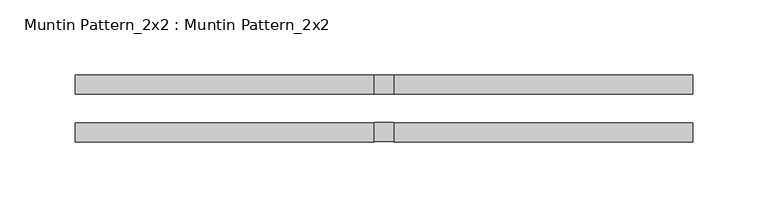
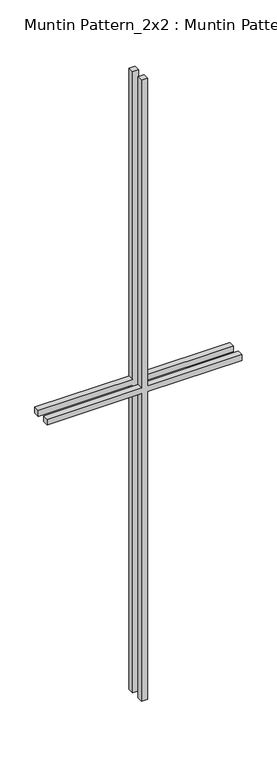
"""IFC4 building model written with IfcOpenShell, lengths in millimetres: proxy geometry, Muntin Pattern_2x2 : Muntin Pattern_2x2."""

from ifc_helpers import new_model, si_unit, frame, origin, place, context, project, spatial, polyline, outline, extrude, source, transform, mapped, element, save


def muntin_pattern_2x2_muntin_pattern_2x2_63bd3b25(model_context):
    return source(origin(), model_context, "Body", "SweptSolid", [
        extrude(outline(polyline([(698.5, -6.35), (698.5, -205.5885801), (685.8, -205.5885801), (685.8, -6.35), (0.0, -6.35), (0.0, 6.35), (685.8, 6.35), (685.8, 205.5885801), (698.5, 205.5885801), (698.5, 6.35), (1384.3, 6.35), (1384.3, -6.35), (698.5, -6.35)])), frame((0.0, 9.525, 0.0), z_axis=(0.0, 1.0, 0.0), x_axis=(0.0, 0.0, 1.0)), (0.0, 0.0, 1.0), 12.7),
        extrude(outline(polyline([(698.5, -6.35), (698.5, -205.5885801), (685.8, -205.5885801), (685.8, -6.35), (0.0, -6.35), (0.0, 6.35), (685.8, 6.35), (685.8, 205.5885801), (698.5, 205.5885801), (698.5, 6.35), (1384.3, 6.35), (1384.3, -6.35), (698.5, -6.35)])), frame((0.0, -22.225, 0.0), z_axis=(0.0, 1.0, 0.0), x_axis=(0.0, 0.0, 1.0)), (0.0, 0.0, 1.0), 12.7),
    ])


if __name__ == "__main__":
    model = new_model("IFC4")
    model_context = context("Model", 3, world=origin())
    ifc_project = project(units=[si_unit("LENGTHUNIT", "METRE", prefix="MILLI")], contexts=[model_context])
    site = spatial("IfcSite", under=ifc_project)
    building = spatial("IfcBuilding", under=site)
    placement = place(None, origin())
    muntin_pattern_2x2_muntin_pattern_2x2_shape = muntin_pattern_2x2_muntin_pattern_2x2_63bd3b25(model_context)
    element("IfcBuildingElementProxy", 1, Name="Muntin Pattern_2x2 : Muntin Pattern_2x2", ObjectType="Muntin Pattern_2x2 : Muntin Pattern_2x2", at=placement, inside=building, context=model_context, shape_type="MappedRepresentation", body=[
        mapped(muntin_pattern_2x2_muntin_pattern_2x2_shape, transform((0.0, 0.0, 0.0), x_axis=(1.0, 0.0, 0.0), y_axis=(0.0, 1.0, 0.0), z_axis=(0.0, 0.0, 1.0))),
    ])
    save(model, "model.ifc")

# Revit data of these elements
# Type "Muntin Pattern_2x2 : Muntin Pattern_2x2"
#   Width [instance default] = 4' - 0"
#   Thickness = 0' - 0 1/2"
#   Height [instance default] = 4' - 0"
#   Distance = 0' - 0 3/4"
#   Interior Material [instance default] = none
#   Exterior Material [instance default] = none
#   Default Elevation = 0
# Element 1 (IfcBuildingElementProxy, "Muntin Pattern_2x2 : Muntin Pattern_2x2")
#   Width = 1' - 4.18808"
#   Height = 4' - 6 1/2"
#   Interior Material = Wood - Stained
#   Exterior Material = Clad - White
#   Materials on its faces: "Clad - White", "Wood - Stained"
# Materials
#   "Clad - White": class "Wood", colour RGB 242 242 238, transparency 0, Cost = 0
#   "Wood - Stained": class "Wood", colour RGB 224 178 126, transparency 0, Cost = 0
